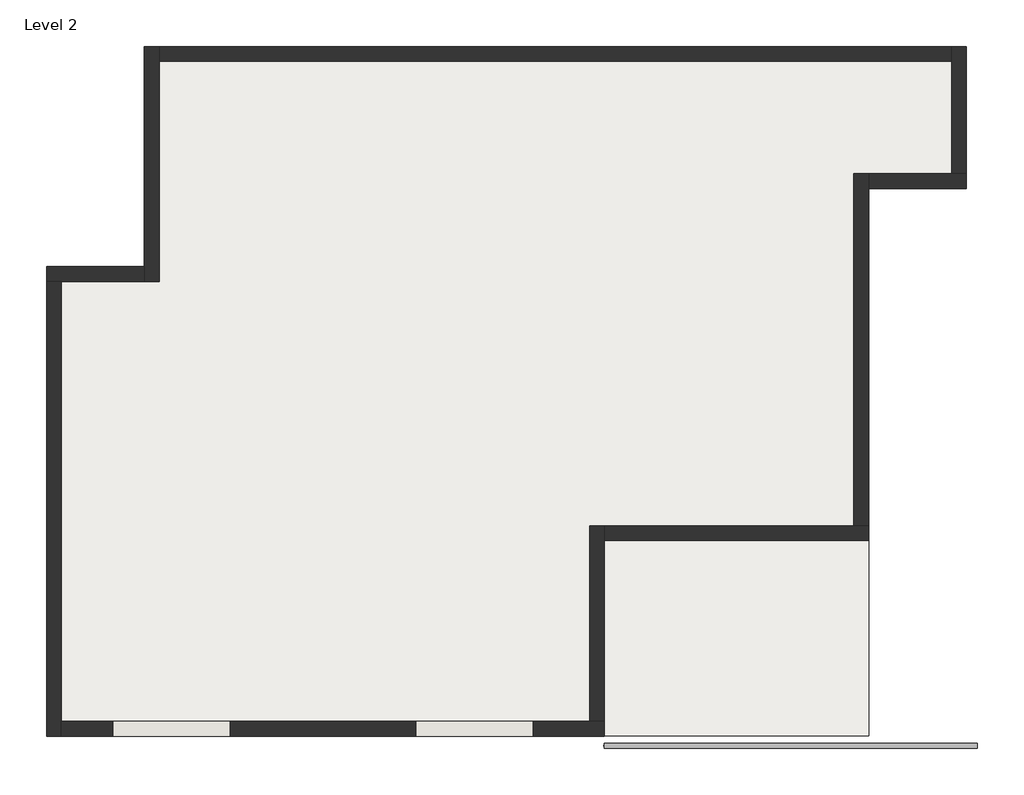
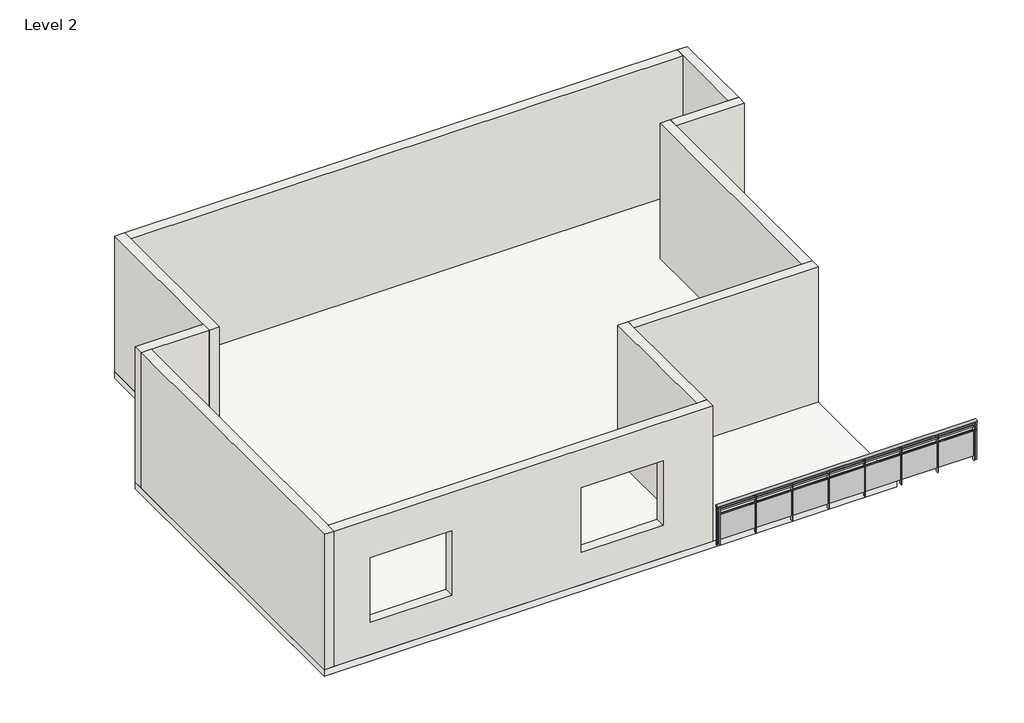
# One storey: 10 walls, 1 railing, 1 slab.
"""IFC4 building model written with IfcOpenShell, lengths in millimetres."""

from ifc_helpers import new_model, si_unit, point, frame, origin, place, context, project, spatial, polyline, ellipse_curve, trimmed, outline, extrude, faceted_brep, element, save
from ifc_brep_helpers import plane_surface, extruded_surface, advanced_brep

model = new_model("IFC4")

# Units and contexts
model_context = context("Model", 3, world=origin())
ifc_project = project(units=[si_unit("LENGTHUNIT", "METRE", prefix="MILLI")], contexts=[model_context])

# Site, building, storey
site = spatial("IfcSite", under=ifc_project)
building = spatial("IfcBuilding", under=site)
storey = spatial("IfcBuildingStorey", under=building, Name="Level 2", Elevation=3048.0)

# Railing
placement = place(None, origin())
element("IfcRailing", 1, ObjectType="Glass Panel - Bottom Fill", at=placement, inside=storey, context=model_context, shape_type="SolidModel", body=[
    advanced_brep(
    [(1099.6319735, 1415.1040735, 3962.4), (1099.6319735, 1338.9040735, 3962.4), (6903.5319735, 1415.1040735, 3962.4), (6903.5319735, 1338.9040735, 3962.4)],
    [
        (0, 1, ellipse_curve(frame((1099.6319735, 1377.0040735, 3962.4), z_axis=(-1.0, 0.0, 0.0), x_axis=(0.0, -1.0, 0.0)), 38.1, 28.575)),
        (1, 0, ellipse_curve(frame((1099.6319735, 1377.0040735, 3962.4), z_axis=(-1.0, 0.0, 0.0), x_axis=(0.0, -1.0, 0.0)), 38.1, 28.575)),
        (2, 3, ellipse_curve(frame((6903.5319735, 1377.0040735, 3962.4), z_axis=(1.0, 0.0, 0.0), x_axis=(0.0, -1.0, 0.0)), 38.1, 28.575)),
        (3, 2, ellipse_curve(frame((6903.5319735, 1377.0040735, 3962.4), z_axis=(1.0, 0.0, 0.0), x_axis=(0.0, -1.0, 0.0)), 38.1, 28.575)),
        (0, 2),
        (3, 1),
    ],
    [
        plane_surface(frame((1099.6319735, 1377.0040735, 3962.4), z_axis=(-1.0, 0.0, 0.0), x_axis=(0.0, 1.0, 0.0))),
        plane_surface(frame((6903.5319735, 1377.0040735, 3962.4), z_axis=(1.0, 0.0, 0.0), x_axis=(0.0, 1.0, 0.0))),
        extruded_surface(trimmed(ellipse_curve(frame((6903.5319735, 1377.0040735, 3962.4), z_axis=(-1.0, 0.0, 0.0), x_axis=(0.0, -1.0, 0.0)), 38.1, 28.575), [point((6903.5319735, 1415.1040735, 3962.4))], [point((6903.5319735, 1338.9040735, 3962.4))], True, "CARTESIAN"), (-5803.900000000001, 0.0, 0.0), 5803.900000000001),
        extruded_surface(trimmed(ellipse_curve(frame((6903.5319735, 1377.0040735, 3962.4), z_axis=(-1.0, 0.0, 0.0), x_axis=(0.0, -1.0, 0.0)), 38.1, 28.575), [point((6903.5319735, 1338.9040735, 3962.4))], [point((6903.5319735, 1415.1040735, 3962.4))], True, "CARTESIAN"), (-5803.900000000001, 0.0, 0.0), 5803.900000000001),
    ],
    [
        (0, [[1, 2]]),
        (1, [[3, 4]]),
        (2, [[-1, 5, -4, 6]]),
        (3, [[-2, -6, -3, -5]]),
    ],
),
    extrude(outline(polyline([(1099.6319735, 1364.3040735), (1099.6319735, 1389.7040735), (6903.5319735, 1389.7040735), (6903.5319735, 1364.3040735), (1099.6319735, 1364.3040735)])), frame((0.0, 0.0, 3848.1), z_axis=(0.0, 0.0, 1.0), x_axis=(1.0, 0.0, 0.0)), (0.0, 0.0, 1.0), 25.4),
    extrude(outline(polyline([(1099.6319735, 1364.3040735), (1099.6319735, 1389.7040735), (6903.5319735, 1389.7040735), (6903.5319735, 1364.3040735), (1099.6319735, 1364.3040735)])), frame((0.0, 0.0, 3746.5), z_axis=(0.0, 0.0, 1.0), x_axis=(1.0, 0.0, 0.0)), (0.0, 0.0, 1.0), 25.4),
    extrude(outline(polyline([(6840.0319735, 1351.6040735), (6840.0319735, 1402.4040735), (6852.7319735, 1402.4040735), (6852.7319735, 1351.6040735), (6840.0319735, 1351.6040735)])), frame((0.0, 0.0, 3048.0), z_axis=(0.0, 0.0, 1.0), x_axis=(1.0, 0.0, 0.0)), (0.0, 0.0, 1.0), 885.825),
    extrude(outline(polyline([(6033.5819735, 1383.5392305), (6846.3819735, 1383.5392305), (6846.3819735, 1377.1892305), (6033.5819735, 1377.1892305), (6033.5819735, 1383.5392305)])), frame((0.0, 0.0, 3149.6), z_axis=(0.0, 0.0, 1.0), x_axis=(1.0, 0.0, 0.0)), (0.0, 0.0, 1.0), 596.9),
    extrude(outline(polyline([(6027.2319735, 1351.6040735), (6027.2319735, 1402.4040735), (6039.9319735, 1402.4040735), (6039.9319735, 1351.6040735), (6027.2319735, 1351.6040735)])), frame((0.0, 0.0, 3048.0), z_axis=(0.0, 0.0, 1.0), x_axis=(1.0, 0.0, 0.0)), (0.0, 0.0, 1.0), 885.825),
    extrude(outline(polyline([(5220.7819735, 1383.5392305), (6033.5819735, 1383.5392305), (6033.5819735, 1377.1892305), (5220.7819735, 1377.1892305), (5220.7819735, 1383.5392305)])), frame((0.0, 0.0, 3149.6), z_axis=(0.0, 0.0, 1.0), x_axis=(1.0, 0.0, 0.0)), (0.0, 0.0, 1.0), 596.9),
    extrude(outline(polyline([(5214.4319735, 1351.6040735), (5214.4319735, 1402.4040735), (5227.1319735, 1402.4040735), (5227.1319735, 1351.6040735), (5214.4319735, 1351.6040735)])), frame((0.0, 0.0, 3048.0), z_axis=(0.0, 0.0, 1.0), x_axis=(1.0, 0.0, 0.0)), (0.0, 0.0, 1.0), 885.825),
    extrude(outline(polyline([(4407.9819735, 1383.5392305), (5220.7819735, 1383.5392305), (5220.7819735, 1377.1892305), (4407.9819735, 1377.1892305), (4407.9819735, 1383.5392305)])), frame((0.0, 0.0, 3149.6), z_axis=(0.0, 0.0, 1.0), x_axis=(1.0, 0.0, 0.0)), (0.0, 0.0, 1.0), 596.9),
    extrude(outline(polyline([(4401.6319735, 1351.6040735), (4401.6319735, 1402.4040735), (4414.3319735, 1402.4040735), (4414.3319735, 1351.6040735), (4401.6319735, 1351.6040735)])), frame((0.0, 0.0, 3048.0), z_axis=(0.0, 0.0, 1.0), x_axis=(1.0, 0.0, 0.0)), (0.0, 0.0, 1.0), 885.825),
    extrude(outline(polyline([(3595.1819735, 1383.5392305), (4407.9819735, 1383.5392305), (4407.9819735, 1377.1892305), (3595.1819735, 1377.1892305), (3595.1819735, 1383.5392305)])), frame((0.0, 0.0, 3149.6), z_axis=(0.0, 0.0, 1.0), x_axis=(1.0, 0.0, 0.0)), (0.0, 0.0, 1.0), 596.9),
    extrude(outline(polyline([(3588.8319735, 1351.6040735), (3588.8319735, 1402.4040735), (3601.5319735, 1402.4040735), (3601.5319735, 1351.6040735), (3588.8319735, 1351.6040735)])), frame((0.0, 0.0, 3048.0), z_axis=(0.0, 0.0, 1.0), x_axis=(1.0, 0.0, 0.0)), (0.0, 0.0, 1.0), 885.825),
    extrude(outline(polyline([(2782.3819735, 1383.5392305), (3595.1819735, 1383.5392305), (3595.1819735, 1377.1892305), (2782.3819735, 1377.1892305), (2782.3819735, 1383.5392305)])), frame((0.0, 0.0, 3149.6), z_axis=(0.0, 0.0, 1.0), x_axis=(1.0, 0.0, 0.0)), (0.0, 0.0, 1.0), 596.9),
    extrude(outline(polyline([(2776.0319735, 1351.6040735), (2776.0319735, 1402.4040735), (2788.7319735, 1402.4040735), (2788.7319735, 1351.6040735), (2776.0319735, 1351.6040735)])), frame((0.0, 0.0, 3048.0), z_axis=(0.0, 0.0, 1.0), x_axis=(1.0, 0.0, 0.0)), (0.0, 0.0, 1.0), 885.825),
    extrude(outline(polyline([(1969.5819735, 1383.5392305), (2782.3819735, 1383.5392305), (2782.3819735, 1377.1892305), (1969.5819735, 1377.1892305), (1969.5819735, 1383.5392305)])), frame((0.0, 0.0, 3149.6), z_axis=(0.0, 0.0, 1.0), x_axis=(1.0, 0.0, 0.0)), (0.0, 0.0, 1.0), 596.9),
    extrude(outline(polyline([(1963.2319735, 1351.6040735), (1963.2319735, 1402.4040735), (1975.9319735, 1402.4040735), (1975.9319735, 1351.6040735), (1963.2319735, 1351.6040735)])), frame((0.0, 0.0, 3048.0), z_axis=(0.0, 0.0, 1.0), x_axis=(1.0, 0.0, 0.0)), (0.0, 0.0, 1.0), 885.825),
    extrude(outline(polyline([(1156.7819735, 1383.5392305), (1969.5819735, 1383.5392305), (1969.5819735, 1377.1892305), (1156.7819735, 1377.1892305), (1156.7819735, 1383.5392305)])), frame((0.0, 0.0, 3149.6), z_axis=(0.0, 0.0, 1.0), x_axis=(1.0, 0.0, 0.0)), (0.0, 0.0, 1.0), 596.9),
    extrude(outline(polyline([(1150.4319735, 1351.6040735), (1150.4319735, 1402.4040735), (1163.1319735, 1402.4040735), (1163.1319735, 1351.6040735), (1150.4319735, 1351.6040735)])), frame((0.0, 0.0, 3048.0), z_axis=(0.0, 0.0, 1.0), x_axis=(1.0, 0.0, 0.0)), (0.0, 0.0, 1.0), 885.825),
    extrude(outline(polyline([(6890.8319735, 1367.4790735), (6890.8319735, 1386.5290735), (6909.8819735, 1386.5290735), (6909.8819735, 1367.4790735), (6890.8319735, 1367.4790735)])), frame((0.0, 0.0, 3048.0), z_axis=(0.0, 0.0, 1.0), x_axis=(1.0, 0.0, 0.0)), (0.0, 0.0, 1.0), 885.825),
    extrude(outline(polyline([(1093.2819735, 1367.4790735), (1093.2819735, 1386.5290735), (1112.3319735, 1386.5290735), (1112.3319735, 1367.4790735), (1093.2819735, 1367.4790735)])), frame((0.0, 0.0, 3048.0), z_axis=(0.0, 0.0, 1.0), x_axis=(1.0, 0.0, 0.0)), (0.0, 0.0, 1.0), 885.825),
])

# Slab
element("IfcSlab", 2, ObjectType="6\"", at=placement, inside=storey, context=model_context, shape_type="SweptSolid", body=[
    extrude(outline(polyline([(-6063.1680265, 12273.6040735), (6738.4319735, 12273.6040735), (6738.4319735, 10063.8040735), (5214.4319735, 10063.8040735), (5214.4319735, 1529.4040735), (-7587.1680265, 1529.4040735), (-7587.1680265, 8844.6040735), (-6063.1680265, 8844.6040735), (-6063.1680265, 12273.6040735)])), frame((0.0, 0.0, 2895.5793129), z_axis=(0.0, 0.0, 1.0), x_axis=(1.0, 0.0, 0.0)), (0.0, 0.0, 1.0), 152.4),
])

# Walls
element("IfcWall", 3, ObjectType="9\" wall", at=placement, inside=storey, context=model_context, shape_type="Brep", body=[
    faceted_brep([(-6063.1680265, 12271.8286055, 3048.0), (-6063.1680265, 8842.8286055, 3048.0), (-6063.1680265, 8614.2286055, 3048.0), (-6063.1680265, 8614.2286055, 6248.4), (-6063.1680265, 8842.8286055, 6248.4), (-6063.1680265, 12271.8286055, 6248.4), (-5834.5680265, 12271.8286055, 3048.0), (-5834.5680265, 12271.8286055, 6248.4), (-5834.5680265, 12043.2286055, 6248.4), (-5834.5680265, 8614.2286055, 6248.4), (-5834.5680265, 8614.2286055, 3048.0), (-5834.5680265, 12043.2286055, 3048.0)], [[[0, 1, 2, 3, 4, 5]], [[6, 7, 8, 9, 10, 11]], [[2, 1, 0, 6, 11, 10]], [[5, 4, 3, 9, 8, 7]], [[3, 2, 10, 9]], [[0, 5, 7, 6]]]),
])
element("IfcWall", 4, ObjectType="9\" wall", at=placement, inside=storey, context=model_context, shape_type="Brep", body=[
    faceted_brep([(-6063.1680265, 8842.8286055, 3048.0), (-7587.1680265, 8842.8286055, 3048.0), (-7587.1680265, 8842.8286055, 6248.4), (-6063.1680265, 8842.8286055, 6248.4), (-6063.1680265, 8614.2286055, 3048.0), (-6063.1680265, 8614.2286055, 6248.4), (-7358.5680265, 8614.2286055, 6248.4), (-7587.1680265, 8614.2286055, 6248.4), (-7587.1680265, 8614.2286055, 3048.0), (-7358.5680265, 8614.2286055, 3048.0)], [[[0, 1, 2, 3]], [[4, 5, 6, 7, 8, 9]], [[1, 0, 4, 9, 8]], [[3, 2, 7, 6, 5]], [[0, 3, 5, 4]], [[2, 1, 8, 7]]]),
])
element("IfcWall", 5, ObjectType="9\" wall", at=placement, inside=storey, context=model_context, shape_type="Brep", body=[
    faceted_brep([(-7587.1680265, 8614.2286055, 3048.0), (-7587.1680265, 1527.6286055, 3048.0), (-7587.1680265, 1527.6286055, 6248.4), (-7587.1680265, 8614.2286055, 6248.4), (-7358.5680265, 8614.2286055, 3048.0), (-7358.5680265, 8614.2286055, 6248.4), (-7358.5680265, 1756.2286055, 6248.4), (-7358.5680265, 1527.6286055, 6248.4), (-7358.5680265, 1527.6286055, 3048.0), (-7358.5680265, 1756.2286055, 3048.0)], [[[0, 1, 2, 3]], [[4, 5, 6, 7, 8, 9]], [[1, 0, 4, 9, 8]], [[3, 2, 7, 6, 5]], [[0, 3, 5, 4]], [[2, 1, 8, 7]]]),
])
element("IfcWall", 6, ObjectType="9\" wall", at=placement, inside=storey, context=model_context, shape_type="Brep", body=[
    faceted_brep([(-7358.5680265, 1527.6286055, 3048.0), (1099.6319735, 1527.6286055, 3048.0), (1099.6319735, 1527.6286055, 6248.4), (-7358.5680265, 1527.6286055, 6248.4), (-6558.4680265, 1527.6286055, 3810.0), (-6558.4680265, 1527.6286055, 5334.0), (-4729.6680265, 1527.6286055, 5334.0), (-4729.6680265, 1527.6286055, 3810.0), (-5.2680265, 1527.6286055, 5334.0), (-5.2680265, 1527.6286055, 3810.0), (-1834.0680265, 1527.6286055, 3810.0), (-1834.0680265, 1527.6286055, 5334.0), (1099.6319735, 1756.2286055, 3048.0), (871.0319735, 1756.2286055, 3048.0), (-7358.5680265, 1756.2286055, 3048.0), (-7358.5680265, 1756.2286055, 6248.4), (871.0319735, 1756.2286055, 6248.4), (1099.6319735, 1756.2286055, 6248.4), (-6558.4680265, 1756.2286055, 5334.0), (-6558.4680265, 1756.2286055, 3810.0), (-4729.6680265, 1756.2286055, 3810.0), (-4729.6680265, 1756.2286055, 5334.0), (-5.2680265, 1756.2286055, 3810.0), (-5.2680265, 1756.2286055, 5334.0), (-1834.0680265, 1756.2286055, 5334.0), (-1834.0680265, 1756.2286055, 3810.0)], [[[0, 1, 2, 3], [4, 5, 6, 7], [8, 9, 10, 11]], [[12, 13, 14, 15, 16, 17], [18, 19, 20, 21], [22, 23, 24, 25]], [[1, 0, 14, 13, 12]], [[3, 2, 17, 16, 15]], [[0, 3, 15, 14]], [[2, 1, 12, 17]], [[18, 5, 4, 19]], [[5, 18, 21, 6]], [[6, 21, 20, 7]], [[19, 4, 7, 20]], [[22, 9, 8, 23]], [[23, 8, 11, 24]], [[24, 11, 10, 25]], [[9, 22, 25, 10]]]),
])
element("IfcWall", 7, ObjectType="9\" wall", at=placement, inside=storey, context=model_context, shape_type="Brep", body=[
    faceted_brep([(1099.6319735, 1756.2286055, 3048.0), (1099.6319735, 4575.6286055, 3048.0), (1099.6319735, 4804.2286055, 3048.0), (1099.6319735, 4804.2286055, 6248.4), (1099.6319735, 4575.6286055, 6248.4), (1099.6319735, 1756.2286055, 6248.4), (871.0319735, 1756.2286055, 3048.0), (871.0319735, 1756.2286055, 6248.4), (871.0319735, 4804.2286055, 6248.4), (871.0319735, 4804.2286055, 3048.0)], [[[0, 1, 2, 3, 4, 5]], [[6, 7, 8, 9]], [[2, 1, 0, 6, 9]], [[5, 4, 3, 8, 7]], [[0, 5, 7, 6]], [[3, 2, 9, 8]]]),
])
element("IfcWall", 8, ObjectType="9\" wall", at=placement, inside=storey, context=model_context, shape_type="Brep", body=[
    faceted_brep([(1099.6319735, 4575.6286055, 3048.0), (5214.4319735, 4575.6286055, 3048.0), (5214.4319735, 4575.6286055, 6248.4), (1099.6319735, 4575.6286055, 6248.4), (1099.6319735, 4804.2286055, 3048.0), (1099.6319735, 4804.2286055, 6248.4), (4985.8319735, 4804.2286055, 6248.4), (5214.4319735, 4804.2286055, 6248.4), (5214.4319735, 4804.2286055, 3048.0), (4985.8319735, 4804.2286055, 3048.0)], [[[0, 1, 2, 3]], [[4, 5, 6, 7, 8, 9]], [[1, 0, 4, 9, 8]], [[3, 2, 7, 6, 5]], [[0, 3, 5, 4]], [[2, 1, 8, 7]]]),
])
element("IfcWall", 9, ObjectType="9\" wall", at=placement, inside=storey, context=model_context, shape_type="Brep", body=[
    faceted_brep([(5214.4319735, 4804.2286055, 3048.0), (5214.4319735, 10062.0286055, 3048.0), (5214.4319735, 10290.6286055, 3048.0), (5214.4319735, 10290.6286055, 6248.4), (5214.4319735, 10062.0286055, 6248.4), (5214.4319735, 4804.2286055, 6248.4), (4985.8319735, 4804.2286055, 3048.0), (4985.8319735, 4804.2286055, 6248.4), (4985.8319735, 10290.6286055, 6248.4), (4985.8319735, 10290.6286055, 3048.0)], [[[0, 1, 2, 3, 4, 5]], [[6, 7, 8, 9]], [[2, 1, 0, 6, 9]], [[5, 4, 3, 8, 7]], [[0, 5, 7, 6]], [[3, 2, 9, 8]]]),
])
element("IfcWall", 10, ObjectType="9\" wall", at=placement, inside=storey, context=model_context, shape_type="Brep", body=[
    faceted_brep([(5214.4319735, 10062.0286055, 3048.0), (6738.4319735, 10062.0286055, 3048.0), (6738.4319735, 10062.0286055, 6248.4), (5214.4319735, 10062.0286055, 6248.4), (5214.4319735, 10290.6286055, 3048.0), (5214.4319735, 10290.6286055, 6248.4), (6509.8319735, 10290.6286055, 6248.4), (6738.4319735, 10290.6286055, 6248.4), (6738.4319735, 10290.6286055, 3048.0), (6509.8319735, 10290.6286055, 3048.0)], [[[0, 1, 2, 3]], [[4, 5, 6, 7, 8, 9]], [[1, 0, 4, 9, 8]], [[3, 2, 7, 6, 5]], [[0, 3, 5, 4]], [[2, 1, 8, 7]]]),
])
element("IfcWall", 11, ObjectType="9\" wall", at=placement, inside=storey, context=model_context, shape_type="Brep", body=[
    faceted_brep([(6738.4319735, 10290.6286055, 3048.0), (6738.4319735, 12271.8286055, 3048.0), (6738.4319735, 12271.8286055, 6248.4), (6738.4319735, 10290.6286055, 6248.4), (6509.8319735, 10290.6286055, 3048.0), (6509.8319735, 10290.6286055, 6248.4), (6509.8319735, 12043.2286055, 6248.4), (6509.8319735, 12271.8286055, 6248.4), (6509.8319735, 12271.8286055, 3048.0), (6509.8319735, 12043.2286055, 3048.0)], [[[0, 1, 2, 3]], [[4, 5, 6, 7, 8, 9]], [[1, 0, 4, 9, 8]], [[3, 2, 7, 6, 5]], [[0, 3, 5, 4]], [[2, 1, 8, 7]]]),
])
element("IfcWall", 12, ObjectType="9\" wall", at=placement, inside=storey, context=model_context, shape_type="SweptSolid", body=[
    extrude(outline(polyline([(-5834.5680265, 12271.8286055), (6509.8319735, 12271.8286055), (6509.8319735, 12043.2286055), (-5834.5680265, 12043.2286055), (-5834.5680265, 12271.8286055)])), frame((0.0, 0.0, 3048.0), z_axis=(0.0, 0.0, 1.0), x_axis=(1.0, 0.0, 0.0)), (0.0, 0.0, 1.0), 3200.4),
])

save(model, "model.ifc")

# Revit data of these elements
# Type "Glass Panel - Bottom Fill"
#   Assembly Code = "C2010400"
#   built-in parameter 1008612 = 0.0416667 (stored number, unit not read)
#   built-in parameter 1008611 = 0.0416667 (stored number, unit not read)
#   built-in parameter 1008609 = 0.333333 (stored number, unit not read)
#   built-in parameter 1008604 = 0.166667 (stored number, unit not read)
#   built-in parameter 1008603 = 0.166667 (stored number, unit not read)
#   Railing Height = 3' - 0"
#   built-in parameter 1008630 = 2
#   built-in parameter 1008610 = 2
#   built-in parameter 1008618 = Baluster - Square : 3/4"
# Type "6\""
#   Assembly Code = "B1010"
#   Function = 0
#   Layers, outside or top first: 0' - 6" "Gypsum Wall Board" (function 1)
# Type "9\" wall"
#   Assembly Code = "B2010"
#   Layers, outside or top first: 0' - 9" "Gypsum Wall Board" (function 1)
# Element 1 (IfcRailing, "Glass Panel - Bottom Fill")
#   Phase Created = New Construction
#   Materials on its faces: "Glass"
# Element 2 (IfcSlab, "6\"")
#   built-in parameter 1001955 = 3.14159 (stored number, unit not read)
#   Height Offset From Level = -0' - 0.00081"
#   Phase Created = New Construction
#   Materials on its faces: "Gypsum Wall Board"
# Elements 3, 4, 5, 6, 7, 8, 9, 10, 11, 12 (IfcWall, "9\" wall")
#   Top Offset = 0' - 0"
#   Base Offset = 0' - 0"
#   wall height = 10' - 6"
#   Phase Created = New Construction
#   Base Constraint = Level 2
#   Top Constraint = Level 4
#   Materials on its faces: "Gypsum Wall Board"
# Materials
#   "Gypsum Wall Board": class "Generic", colour RGB 127 127 127, transparency 0, Description = "Gypsum Wall Board", Cost = 0
#   "Glass": class "Glass", colour RGB 0 128 192, transparency 0.75, Description = "Soda Lime Glass", Cost = 0
